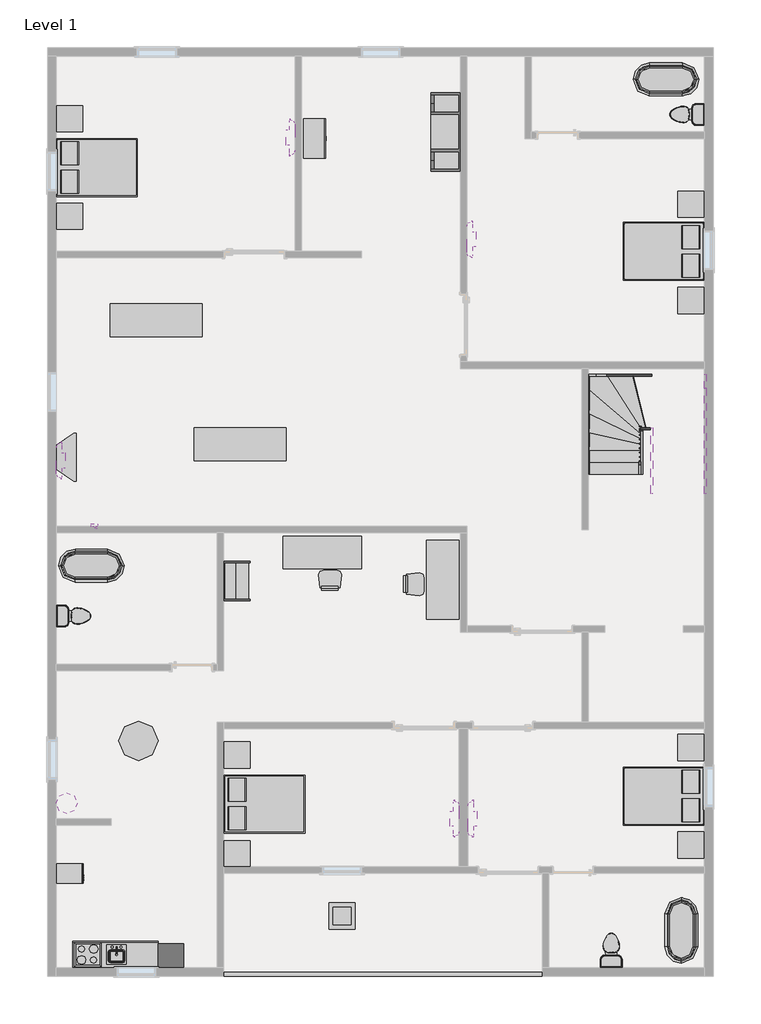
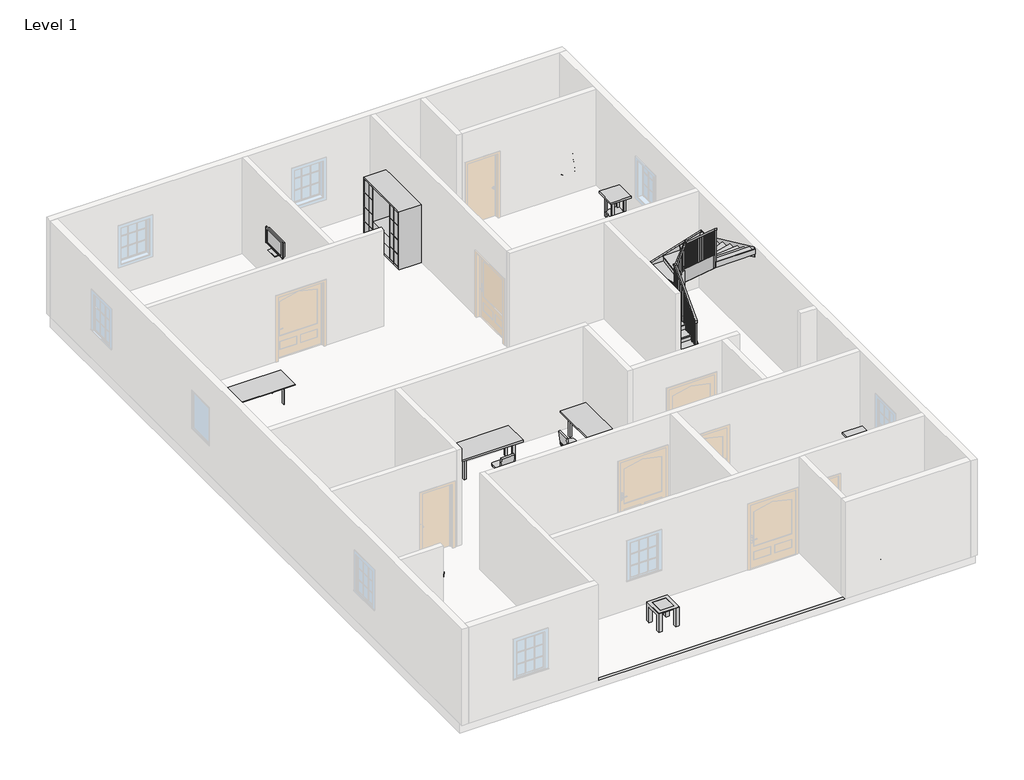
# One storey, part 2 of 2: 29 furniture elements, 9 members, 8 flow terminals, 8 proxies, 1 railing, 1 stair flight.
"""IFC4 building model written with IfcOpenShell, lengths in millimetres."""

from ifc_helpers import new_model, si_unit, frame, origin, place, context, project, spatial, polyline, outline, extrude, faceted_brep, triangles, transform, mapped, element, save
from components import proxy_7e1014cc, proxy_a6faaae8, proxy_45b28599, kitchenette_medium_kitchenette_medium_844211aa, rpc_picture_frame_rpc_picture_frame_c25e3fe9, proxy_c523a7b7, single_carrel_single_carrel_ed4d160c, flow_terminal_871c2e40, flow_terminal_d49f872f, toilet_domestic_3d_toilet_domestic_3d_f7549cf7, toilet_domestic_3d_toilet_domestic_3d_183bbd19, flow_terminal_b374fae2, furniture_c8abb964, chair_desk_chair_desk_ccc35c8f, furniture_c6510c7c, furniture_cf0b6580, furniture_e1dba61b, furniture_56245f3a, tv_stand_tv_stand_6ce107e5, furniture_b5c51a22, furniture_92191dda, furniture_905aceb5, furniture_5bc9ed15, furniture_a5b052b6, stair_flight_8a5f7a69

model = new_model("IFC4")

# Units and contexts
model_context = context("Model", 3, world=origin())
ifc_project = project(units=[si_unit("LENGTHUNIT", "METRE", prefix="MILLI")], contexts=[model_context])

# Site, building, storey
site = spatial("IfcSite", under=ifc_project)
building = spatial("IfcBuilding", under=site)
storey = spatial("IfcBuildingStorey", under=building, Name="Level 1", Elevation=0.0)

# Proxies
placement = place(None, origin())
element("IfcBuildingElementProxy", 1, Name="Building Element Proxy", at=placement, inside=storey, context=model_context, shape_type="Tessellation", body=[
    triangles([(-10823.7858398, -3895.8296448, 0.0), (-10823.7858398, -6283.4298386, 0.0), (-3432.3861305, -6283.4298386, 0.0), (-3432.3861305, -3895.8296448, 0.0)], [[1, 2, 4], [3, 4, 2]], closed=False),
])
proxy_shape = proxy_7e1014cc(model_context)
element("IfcBuildingElementProxy", 2, Name="18\" x 24\" x 34 1/2\"", ObjectType="18\" x 24\" x 34 1/2\"", at=placement, inside=storey, context=model_context, shape_type="MappedRepresentation", body=[
    mapped(proxy_shape, transform((-14138.7364865, -4201.9470633, 0.0), x_axis=(0.0, 1.0, 0.0), y_axis=(-1.0, 0.0, 0.0), z_axis=(0.0, 0.0, 1.0))),
])
proxy_2_shape = proxy_a6faaae8(model_context)
element("IfcBuildingElementProxy", 3, Name="Cook Top-4 Unit2 : 22\" x 20\"", ObjectType="Cook Top-4 Unit2 : 22\" x 20\"", at=placement, inside=storey, context=model_context, shape_type="MappedRepresentation", body=[
    mapped(proxy_2_shape, transform((-13986.0860513, -5775.4295948, 0.0), x_axis=(1.0, 0.0, 0.0), y_axis=(0.0, 1.0, 0.0), z_axis=(0.0, 0.0, 1.0))),
])
proxy_3_shape = proxy_45b28599(model_context)
element("IfcBuildingElementProxy", 4, Name="Dishwasher : 24\" x 24\" x 34\"", ObjectType="Dishwasher : 24\" x 24\" x 34\"", at=placement, inside=storey, context=model_context, shape_type="MappedRepresentation", body=[
    mapped(proxy_3_shape, transform((-13034.9035198, -6067.2791596, 0.0), x_axis=(1.0, 0.0, 0.0), y_axis=(0.0, 1.0, 0.0), z_axis=(0.0, 0.0, 1.0))),
])
kitchenette_medium_kitchenette_medium_shape = kitchenette_medium_kitchenette_medium_844211aa(model_context)
element("IfcBuildingElementProxy", 5, Name="Kitchenette - Medium : Kitchenette - Medium", ObjectType="Kitchenette - Medium : Kitchenette - Medium", at=placement, inside=storey, context=model_context, shape_type="MappedRepresentation", body=[
    mapped(kitchenette_medium_kitchenette_medium_shape, transform((-13661.9237562, -5470.6295948, 0.0), x_axis=(1.0, 0.0, 0.0), y_axis=(0.0, 1.0, 0.0), z_axis=(0.0, 0.0, 1.0))),
])
rpc_picture_frame_rpc_picture_frame_shape = rpc_picture_frame_rpc_picture_frame_c25e3fe9(model_context)
element("IfcBuildingElementProxy", 6, Name="RPC Picture Frame : RPC Picture Frame", ObjectType="RPC Picture Frame : RPC Picture Frame", at=placement, inside=storey, context=model_context, shape_type="MappedRepresentation", body=[
    mapped(rpc_picture_frame_rpc_picture_frame_shape, transform((-13828.5359953, 4155.9704052, 2133.6), x_axis=(-1.0000000000000004, 0.0, 0.0), y_axis=(0.0, -1.0000000000000004, 0.0), z_axis=(0.0, 0.0, 1.0))),
])
proxy_4_shape = proxy_c523a7b7(model_context)
element("IfcBuildingElementProxy", 7, Name="Refrigerator : 24\" x 25\" LH", ObjectType="Refrigerator : 24\" x 25\" LH", at=placement, inside=storey, context=model_context, shape_type="MappedRepresentation", body=[
    mapped(proxy_4_shape, transform((-12049.3360513, -5821.0785663, 0.0), x_axis=(1.0, 0.0, 0.0), y_axis=(0.0, 1.0, 0.0), z_axis=(0.0, 0.0, 1.0))),
])
single_carrel_single_carrel_shape = single_carrel_single_carrel_ed4d160c(model_context)
element("IfcBuildingElementProxy", 8, Name="Single Carrel : Single Carrel", ObjectType="Single Carrel : Single Carrel", at=placement, inside=storey, context=model_context, shape_type="MappedRepresentation", body=[
    mapped(single_carrel_single_carrel_shape, transform((-10823.7860513, 2885.9704052, 0.0), x_axis=(0.0, 1.0000000000000002, 0.0), y_axis=(-1.0000000000000002, 0.0, 0.0), z_axis=(0.0, 0.0, 1.0))),
])

# Flow terminals
flow_terminal_shape = flow_terminal_871c2e40(model_context)
element("IfcFlowTerminal", 9, ObjectType="Sink Kitchen-Island : 18\" x 18\"", at=placement, inside=storey, context=model_context, shape_type="MappedRepresentation", body=[
    mapped(flow_terminal_shape, transform((-13328.6752918, -5777.7749959, -14.4), x_axis=(1.0, 0.0, 0.0), y_axis=(0.0, 1.0, 0.0), z_axis=(0.0, 0.0, 1.0))),
])
flow_terminal_2_shape = flow_terminal_d49f872f(model_context)
element("IfcFlowTerminal", 10, ObjectType="Sink Vanity-Round : 19\" x 19\"", at=placement, inside=storey, context=model_context, shape_type="MappedRepresentation", body=[
    mapped(flow_terminal_2_shape, transform((-14385.2142446, -2366.8813354, 914.4), x_axis=(0.0, 1.0000000000000002, 0.0), y_axis=(-1.0000000000000002, 0.0, 0.0), z_axis=(0.0, 0.0, 1.0))),
])
toilet_domestic_3d_toilet_domestic_3d_shape = toilet_domestic_3d_toilet_domestic_3d_f7549cf7(model_context)
toilet_domestic_3d_toilet_domestic_3d_2_shape = toilet_domestic_3d_toilet_domestic_3d_183bbd19(model_context)
element("IfcFlowTerminal", 11, ObjectType="Toilet-Domestic-3D : Toilet-Domestic-3D", at=placement, inside=storey, context=model_context, shape_type="MappedRepresentation", body=[
    mapped(toilet_domestic_3d_toilet_domestic_3d_shape, transform((-1832.1860513, -5585.5335675, 0.0), x_axis=(-1.0000000000000004, 0.0, 0.0), y_axis=(0.0, -1.0000000000000004, 0.0), z_axis=(0.0, 0.0, 1.0))),
    mapped(toilet_domestic_3d_toilet_domestic_3d_2_shape, transform((-1832.1860513, -5585.5335675, 0.0), x_axis=(-1.0000000000000004, 0.0, 0.0), y_axis=(0.0, -1.0000000000000004, 0.0), z_axis=(0.0, 0.0, 1.0))),
])
element("IfcFlowTerminal", 12, ObjectType="Toilet-Domestic-3D : Toilet-Domestic-3D", at=placement, inside=storey, context=model_context, shape_type="MappedRepresentation", body=[
    mapped(toilet_domestic_3d_toilet_domestic_3d_shape, transform((-167.8820786, 13706.3704052, 0.0), x_axis=(0.0, -1.0000000000000002, 0.0), y_axis=(1.0000000000000002, 0.0, 0.0), z_axis=(0.0, 0.0, 1.0))),
    mapped(toilet_domestic_3d_toilet_domestic_3d_2_shape, transform((-167.8820786, 13706.3704052, 0.0), x_axis=(0.0, -1.0000000000000002, 0.0), y_axis=(1.0000000000000002, 0.0, 0.0), z_axis=(0.0, 0.0, 1.0))),
])
element("IfcFlowTerminal", 13, ObjectType="Toilet-Domestic-3D : Toilet-Domestic-3D", at=placement, inside=storey, context=model_context, shape_type="MappedRepresentation", body=[
    mapped(toilet_domestic_3d_toilet_domestic_3d_shape, transform((-14215.2900239, 2073.1704052, 0.0), x_axis=(0.0, 1.0000000000000002, 0.0), y_axis=(-1.0000000000000002, 0.0, 0.0), z_axis=(0.0, 0.0, 1.0))),
    mapped(toilet_domestic_3d_toilet_domestic_3d_2_shape, transform((-14215.2900239, 2073.1704052, 0.0), x_axis=(0.0, 1.0000000000000002, 0.0), y_axis=(-1.0000000000000002, 0.0, 0.0), z_axis=(0.0, 0.0, 1.0))),
])
flow_terminal_3_shape = flow_terminal_b374fae2(model_context)
element("IfcFlowTerminal", 14, ObjectType="Tub-Free Standing-3D : 30\" x 60\"", at=placement, inside=storey, context=model_context, shape_type="MappedRepresentation", body=[
    mapped(flow_terminal_3_shape, transform((-206.5860513, -5216.6295948, 0.0), x_axis=(-1.0000000000000004, 0.0, 0.0), y_axis=(0.0, -1.0000000000000004, 0.0), z_axis=(0.0, 0.0, 1.0))),
])
element("IfcFlowTerminal", 15, ObjectType="Tub-Free Standing-3D : 30\" x 60\"", at=placement, inside=storey, context=model_context, shape_type="MappedRepresentation", body=[
    mapped(flow_terminal_3_shape, transform((-13897.1860513, 3241.5704052, 0.0), x_axis=(0.0, 1.0000000000000004, 0.0), y_axis=(-1.0000000000000004, 0.0, 0.0), z_axis=(0.0, 0.0, 1.0))),
])
element("IfcFlowTerminal", 16, ObjectType="Tub-Free Standing-3D : 30\" x 60\"", at=placement, inside=storey, context=model_context, shape_type="MappedRepresentation", body=[
    mapped(flow_terminal_3_shape, transform((-562.1860513, 14519.1704052, 0.0), x_axis=(0.0, -1.0000000000000004, 0.0), y_axis=(1.0000000000000004, 0.0, 0.0), z_axis=(0.0, 0.0, 1.0))),
])

# Furniture
furniture_shape = furniture_c8abb964(model_context)
element("IfcFurniture", 17, ObjectType="Bed-Box : Double 53\" x 74\"", at=placement, inside=storey, context=model_context, shape_type="MappedRepresentation", body=[
    mapped(furniture_shape, transform((-10118.4155595, -2625.8295948, 0.0), x_axis=(0.0, 1.0, 0.0), y_axis=(-1.0, 0.0, 0.0), z_axis=(0.0, 0.0, 1.0))),
])
element("IfcFurniture", 18, ObjectType="Bed-Box : Double 53\" x 74\"", at=placement, inside=storey, context=model_context, shape_type="MappedRepresentation", body=[
    mapped(furniture_shape, transform((-378.5565431, -1765.9771358, 0.0), x_axis=(0.0, -1.0000000000000004, 0.0), y_axis=(1.0000000000000004, 0.0, 0.0), z_axis=(0.0, 0.0, 1.0))),
])
element("IfcFurniture", 19, ObjectType="Bed-Box : Double 53\" x 74\"", at=placement, inside=storey, context=model_context, shape_type="MappedRepresentation", body=[
    mapped(furniture_shape, transform((-14004.6155595, 12135.3179462, 0.0), x_axis=(0.0, 1.0000000000000007, 0.0), y_axis=(-1.0000000000000007, 0.0, 0.0), z_axis=(0.0, 0.0, 1.0))),
])
element("IfcFurniture", 20, ObjectType="Bed-Box : Double 53\" x 74\"", at=placement, inside=storey, context=model_context, shape_type="MappedRepresentation", body=[
    mapped(furniture_shape, transform((-378.5565431, 10870.5228642, 0.0), x_axis=(0.0, -1.0000000000000004, 0.0), y_axis=(1.0000000000000004, 0.0, 0.0), z_axis=(0.0, 0.0, 1.0))),
])
chair_desk_chair_desk_shape = chair_desk_chair_desk_ccc35c8f(model_context)
element("IfcFurniture", 21, ObjectType="Chair-Desk : Chair-Desk", at=placement, inside=storey, context=model_context, shape_type="MappedRepresentation", body=[
    mapped(chair_desk_chair_desk_shape, transform((-8359.9860513, 2733.5704052, 0.0), x_axis=(1.0, 0.0, 0.0), y_axis=(0.0, 1.0, 0.0), z_axis=(0.0, 0.0, 1.0))),
])
element("IfcFurniture", 22, ObjectType="Chair-Desk : Chair-Desk", at=placement, inside=storey, context=model_context, shape_type="MappedRepresentation", body=[
    mapped(chair_desk_chair_desk_shape, transform((-6581.9860513, 2809.7704052, 0.0), x_axis=(0.0, -1.0000000000000004, 0.0), y_axis=(1.0000000000000004, 0.0, 0.0), z_axis=(0.0, 0.0, 1.0))),
])
furniture_2_shape = furniture_c6510c7c(model_context)
element("IfcFurniture", 23, ObjectType="Counter Top w Sink Hole : 24\" Depth", at=placement, inside=storey, context=model_context, shape_type="MappedRepresentation", body=[
    mapped(furniture_2_shape, transform((-13128.5237562, -5470.6295948, -14.4), x_axis=(1.0, 0.0, 0.0), y_axis=(0.0, 1.0, 0.0), z_axis=(0.0, 0.0, 1.0))),
])
furniture_3_shape = furniture_cf0b6580(model_context)
element("IfcFurniture", 24, ObjectType="Entertainment Center : 72\" x 72\" x 24\"", at=placement, inside=storey, context=model_context, shape_type="MappedRepresentation", body=[
    mapped(furniture_3_shape, transform((-5235.7860513, 13299.9704052, 0.0), x_axis=(0.0, -1.0000000000000007, 0.0), y_axis=(1.0000000000000007, 0.0, 0.0), z_axis=(0.0, 0.0, 1.0))),
])
furniture_4_shape = furniture_e1dba61b(model_context)
element("IfcFurniture", 25, ObjectType="Storage Pedestal : 20\" x 36\" x 36\"", at=placement, inside=storey, context=model_context, shape_type="MappedRepresentation", body=[
    mapped(furniture_4_shape, transform((-9649.9044273, 13327.5929191, 0.0), x_axis=(0.0, 1.0000000000000009, 0.0), y_axis=(-1.0000000000000009, 0.0, 0.0), z_axis=(0.0, 0.0, 1.0))),
])
furniture_5_shape = furniture_56245f3a(model_context)
element("IfcFurniture", 26, ObjectType="TV - Flat Screen : 32\"", at=placement, inside=storey, context=model_context, shape_type="MappedRepresentation", body=[
    mapped(furniture_5_shape, transform((-14651.4474276, 5683.9149193, 1524.0), x_axis=(0.0, 1.0000000000000002, 0.0), y_axis=(-1.0000000000000002, 0.0, 0.0), z_axis=(0.0, 0.0, 1.0))),
])
element("IfcFurniture", 27, ObjectType="TV - Flat Screen : 32\"", at=placement, inside=storey, context=model_context, shape_type="MappedRepresentation", body=[
    mapped(furniture_5_shape, transform((-5101.0474276, -2621.8850807, 1219.2), x_axis=(0.0, 1.0000000000000002, 0.0), y_axis=(-1.0000000000000002, 0.0, 0.0), z_axis=(0.0, 0.0, 1.0))),
])
element("IfcFurniture", 28, ObjectType="TV - Flat Screen : 32\"", at=placement, inside=storey, context=model_context, shape_type="MappedRepresentation", body=[
    mapped(furniture_5_shape, transform((-5421.3246749, -2629.774109, 1219.2), x_axis=(0.0, -1.0000000000000002, 0.0), y_axis=(1.0000000000000002, 0.0, 0.0), z_axis=(0.0, 0.0, 1.0))),
])
element("IfcFurniture", 29, ObjectType="TV - Flat Screen : 32\"", at=placement, inside=storey, context=model_context, shape_type="MappedRepresentation", body=[
    mapped(furniture_5_shape, transform((-5126.4474276, 10814.7149193, 1219.2), x_axis=(0.0, 1.0000000000000002, 0.0), y_axis=(-1.0000000000000002, 0.0, 0.0), z_axis=(0.0, 0.0, 1.0))),
])
element("IfcFurniture", 30, ObjectType="TV - Flat Screen : 32\"", at=placement, inside=storey, context=model_context, shape_type="MappedRepresentation", body=[
    mapped(furniture_5_shape, transform((-9231.3246749, 13169.025891, 1219.2), x_axis=(0.0, -1.0000000000000004, 0.0), y_axis=(1.0000000000000004, 0.0, 0.0), z_axis=(0.0, 0.0, 1.0))),
])
tv_stand_tv_stand_shape = tv_stand_tv_stand_6ce107e5(model_context)
element("IfcFurniture", 31, ObjectType="TV Stand : TV Stand", at=placement, inside=storey, context=model_context, shape_type="MappedRepresentation", body=[
    mapped(tv_stand_tv_stand_shape, transform((-14709.9860513, 5630.9824031, 0.0), x_axis=(0.0, 1.0000000000000002, 0.0), y_axis=(-1.0000000000000002, 0.0, 0.0), z_axis=(0.0, 0.0, 1.0))),
])
furniture_6_shape = furniture_b5c51a22(model_context)
element("IfcFurniture", 32, ObjectType="Table-Coffee : 24\" x 24\" x 24\"", at=placement, inside=storey, context=model_context, shape_type="MappedRepresentation", body=[
    mapped(furniture_6_shape, transform((-8098.8518179, -4981.6406726, 0.0), x_axis=(1.0, 0.0, 0.0), y_axis=(0.0, 1.0, 0.0), z_axis=(0.0, 0.0, 1.0))),
])
furniture_7_shape = furniture_92191dda(model_context)
element("IfcFurniture", 33, ObjectType="Table-Dining : 30\" x 84\" x 22\"", at=placement, inside=storey, context=model_context, shape_type="MappedRepresentation", body=[
    mapped(furniture_7_shape, transform((-10461.0518179, 5965.7593274, 0.0), x_axis=(1.0, 0.0, 0.0), y_axis=(0.0, 1.0, 0.0), z_axis=(0.0, 0.0, 1.0))),
])
element("IfcFurniture", 34, ObjectType="Table-Dining : 30\" x 84\" x 22\"", at=placement, inside=storey, context=model_context, shape_type="MappedRepresentation", body=[
    mapped(furniture_7_shape, transform((-12416.8518179, 8835.9593274, 0.0), x_axis=(1.0, 0.0, 0.0), y_axis=(0.0, 1.0, 0.0), z_axis=(0.0, 0.0, 1.0))),
])
furniture_8_shape = furniture_905aceb5(model_context)
element("IfcFurniture", 35, ObjectType="Table-Dining Round w Chairs : 36\" Diameter", at=placement, inside=storey, context=model_context, shape_type="MappedRepresentation", body=[
    mapped(furniture_8_shape, transform((-12908.6680185, -637.5509063, 0.0), x_axis=(1.0, 0.0, 0.0), y_axis=(0.0, 1.0, 0.0), z_axis=(0.0, 0.0, 1.0))),
])
furniture_9_shape = furniture_5bc9ed15(model_context)
element("IfcFurniture", 36, ObjectType="Table-Night Stand : 24\" x 24\" x 30\"", at=placement, inside=storey, context=model_context, shape_type="MappedRepresentation", body=[
    mapped(furniture_9_shape, transform((-10827.5196816, -3743.4295948, 0.0), x_axis=(1.0, 0.0, 0.0), y_axis=(0.0, 1.0, 0.0), z_axis=(0.0, 0.0, 1.0))),
])
element("IfcFurniture", 37, ObjectType="Table-Night Stand : 24\" x 24\" x 30\"", at=placement, inside=storey, context=model_context, shape_type="MappedRepresentation", body=[
    mapped(furniture_9_shape, transform((-10827.5196816, -1457.4295948, 0.0), x_axis=(1.0, 0.0, 0.0), y_axis=(0.0, 1.0, 0.0), z_axis=(0.0, 0.0, 1.0))),
])
element("IfcFurniture", 38, ObjectType="Table-Night Stand : 24\" x 24\" x 30\"", at=placement, inside=storey, context=model_context, shape_type="MappedRepresentation", body=[
    mapped(furniture_9_shape, transform((-286.5196816, -3540.2295948, 0.0), x_axis=(1.0, 0.0, 0.0), y_axis=(0.0, 1.0, 0.0), z_axis=(0.0, 0.0, 1.0))),
])
element("IfcFurniture", 39, ObjectType="Table-Night Stand : 24\" x 24\" x 30\"", at=placement, inside=storey, context=model_context, shape_type="MappedRepresentation", body=[
    mapped(furniture_9_shape, transform((-286.5196816, -1279.6295948, 0.0), x_axis=(1.0, 0.0, 0.0), y_axis=(0.0, 1.0, 0.0), z_axis=(0.0, 0.0, 1.0))),
])
element("IfcFurniture", 40, ObjectType="Table-Night Stand : 24\" x 24\" x 30\"", at=placement, inside=storey, context=model_context, shape_type="MappedRepresentation", body=[
    mapped(furniture_9_shape, transform((-286.5196816, 11318.7704052, 0.0), x_axis=(1.0, 0.0, 0.0), y_axis=(0.0, 1.0, 0.0), z_axis=(0.0, 0.0, 1.0))),
])
element("IfcFurniture", 41, ObjectType="Table-Night Stand : 24\" x 24\" x 30\"", at=placement, inside=storey, context=model_context, shape_type="MappedRepresentation", body=[
    mapped(furniture_9_shape, transform((-286.5196816, 9083.5704052, 0.0), x_axis=(1.0, 0.0, 0.0), y_axis=(0.0, 1.0, 0.0), z_axis=(0.0, 0.0, 1.0))),
])
element("IfcFurniture", 42, ObjectType="Table-Night Stand : 24\" x 24\" x 30\"", at=placement, inside=storey, context=model_context, shape_type="MappedRepresentation", body=[
    mapped(furniture_9_shape, transform((-14713.7196816, 13299.9704052, 0.0), x_axis=(1.0, 0.0, 0.0), y_axis=(0.0, 1.0, 0.0), z_axis=(0.0, 0.0, 1.0))),
])
element("IfcFurniture", 43, ObjectType="Table-Night Stand : 24\" x 24\" x 30\"", at=placement, inside=storey, context=model_context, shape_type="MappedRepresentation", body=[
    mapped(furniture_9_shape, transform((-14713.7196816, 11039.3704052, 0.0), x_axis=(1.0, 0.0, 0.0), y_axis=(0.0, 1.0, 0.0), z_axis=(0.0, 0.0, 1.0))),
])
furniture_10_shape = furniture_a5b052b6(model_context)
element("IfcFurniture", 44, ObjectType="Table-Rectangular : 72\" x 30\"", at=placement, inside=storey, context=model_context, shape_type="MappedRepresentation", body=[
    mapped(furniture_10_shape, transform((-8537.7860513, 3546.3704052, 0.0), x_axis=(1.0, 0.0, 0.0), y_axis=(0.0, 1.0, 0.0), z_axis=(0.0, 0.0, 1.0))),
])
element("IfcFurniture", 45, ObjectType="Table-Rectangular : 72\" x 30\"", at=placement, inside=storey, context=model_context, shape_type="MappedRepresentation", body=[
    mapped(furniture_10_shape, transform((-5743.7860513, 2911.3704052, 0.0), x_axis=(0.0, -1.0000000000000004, 0.0), y_axis=(1.0000000000000004, 0.0, 0.0), z_axis=(0.0, 0.0, 1.0))),
])

# Members
element("IfcMember", 46, ObjectType="Stringer - 2\" Width", at=placement, inside=storey, context=model_context, shape_type="SweptSolid", body=[
    extrude(outline(polyline([(5356.2607598, 0.0), (5356.2607598, 253.7697654), (7536.5486445, 1127.7715314), (7536.5486445, 799.3938411), (5542.377952, 0.0), (5356.2607598, 0.0)])), frame((-2389.7053008, 0.0, 0.0), z_axis=(1.0, 0.0, 0.0), x_axis=(0.0, 1.0, 0.0)), (0.0, 0.0, 1.0), 50.8),
])
element("IfcMember", 47, ObjectType="Stringer - 2\" Width", at=placement, inside=storey, context=model_context, shape_type="SweptSolid", body=[
    extrude(outline(polyline([(-2338.9053008, 7536.5486445), (-2389.7053008, 7536.5486445), (-2389.7053008, 7685.2896548), (-2338.9053008, 7634.4896548), (-2338.9053008, 7536.5486445)])), frame((0.0, 0.0, 799.3938411), z_axis=(0.0, 0.0, 1.0), x_axis=(1.0, 0.0, 0.0)), (0.0, 0.0, 1.0), 328.3776903),
])
element("IfcMember", 48, ObjectType="Stringer - 2\" Width", at=placement, inside=storey, context=model_context, shape_type="SweptSolid", body=[
    extrude(outline(polyline([(-2338.9053008, 7634.4896548), (-2389.7053008, 7685.2896548), (-2181.2813511, 7685.2896548), (-2181.2813511, 7634.4896548), (-2338.9053008, 7634.4896548)])), frame((0.0, 0.0, 799.3938411), z_axis=(0.0, 0.0, 1.0), x_axis=(1.0, 0.0, 0.0)), (0.0, 0.0, 1.0), 328.3776903),
])
element("IfcMember", 49, ObjectType="Stringer - 2\" Width", at=placement, inside=storey, context=model_context, shape_type="SweptSolid", body=[
    extrude(outline(polyline([(1127.7715314, -2181.2813511), (799.3938411, -2181.2813511), (1575.7906145, 325.5331983), (1899.7048199, 325.5331983), (1899.7048199, 311.1215864), (1127.7715314, -2181.2813511)])), frame((0.0, 7634.4896548, 0.0), z_axis=(0.0, 1.0, 0.0), x_axis=(0.0, 0.0, 1.0)), (0.0, 0.0, 1.0), 50.8),
])
element("IfcMember", 50, ObjectType="Stringer - 2\" Width", at=placement, inside=storey, context=model_context, shape_type="SweptSolid", body=[
    extrude(outline(polyline([(325.5331983, 7685.2896548), (376.3331983, 7685.2896548), (376.3331983, 7355.703067), (325.5331983, 7355.703067), (325.5331983, 7685.2896548)])), frame((0.0, 0.0, 1580.6208435), z_axis=(0.0, 0.0, 1.0), x_axis=(1.0, 0.0, 0.0)), (0.0, 0.0, 1.0), 319.0839764),
])
element("IfcMember", 51, ObjectType="Stringer - 2\" Width", at=placement, inside=storey, context=model_context, shape_type="SweptSolid", body=[
    extrude(outline(polyline([(5356.2607598, 0.0), (5356.2607598, 140.6708409), (6391.1704052, 1235.2332807), (6391.1704052, 791.5839653), (5642.7271451, 0.0), (5356.2607598, 0.0)])), frame((-1146.3860513, 0.0, 0.0), z_axis=(1.0, 0.0, 0.0), x_axis=(0.0, 1.0, 0.0)), (0.0, 0.0, 1.0), 50.8),
])
element("IfcMember", 52, ObjectType="Stringer - 2\" Width", at=placement, inside=storey, context=model_context, shape_type="SweptSolid", body=[
    extrude(outline(polyline([(1453.6314878, -1146.3860513), (845.3121069, -1146.3860513), (845.3121069, -1087.3182945), (1219.5911959, -917.7860513), (1835.3677632, -917.7860513), (1835.3677632, -973.4760251), (1453.6314878, -1146.3860513)])), frame((0.0, 6391.1704052, 0.0), z_axis=(0.0, 1.0, 0.0), x_axis=(0.0, 0.0, 1.0)), (0.0, 0.0, 1.0), 50.8),
])
element("IfcMember", 53, ObjectType="Stringer - 2\" Width", at=placement, inside=storey, context=model_context, shape_type="SweptSolid", body=[
    extrude(outline(polyline([(6441.9704052, 1835.3677632), (6441.9704052, 1426.0789229), (4914.2387133, 2795.2042452), (4914.2387133, 3204.4930856), (6441.9704052, 1835.3677632)])), frame((-917.7860513, 0.0, 0.0), z_axis=(1.0, 0.0, 0.0), x_axis=(0.0, 1.0, 0.0)), (0.0, 0.0, 1.0), 50.8),
])
element("IfcMember", 54, ObjectType="Stringer - 2\" Width", at=placement, inside=storey, context=model_context, shape_type="SweptSolid", body=[
    extrude(outline(polyline([(7355.703067, 1899.7048199), (7355.703067, 1580.6208435), (4914.2387133, 2711.6595982), (4914.2387133, 3030.7435746), (7355.703067, 1899.7048199)])), frame((325.5331983, 0.0, 0.0), z_axis=(1.0, 0.0, 0.0), x_axis=(0.0, 1.0, 0.0)), (0.0, 0.0, 1.0), 50.8),
])

# Railing
element("IfcRailing", 55, ObjectType="Handrail - Rectangular", at=placement, inside=storey, context=model_context, shape_type="SolidModel", body=[
    faceted_brep([(-1197.1860513, 5356.2607598, 957.561888), (-1197.1860513, 5356.2607598, 883.6203354), (-1146.3860513, 5356.2607598, 883.6203354), (-1146.3860513, 5356.2607598, 957.561888), (-1197.1860513, 6412.8357789, 2075.0385063), (-1197.1860513, 6434.716135, 2024.2385063), (-1146.3860513, 6434.716135, 2024.2385063), (-1146.3860513, 6412.8357789, 2075.0385063), (-1197.1860513, 6492.7704052, 2075.0385063), (-1146.3860513, 6492.7704052, 2075.0385063), (-1146.3860513, 6492.7704052, 2024.2385063), (-1197.1860513, 6492.7704052, 2024.2385063)], [[[0, 1, 2, 3]], [[1, 0, 4, 5]], [[2, 1, 5, 6]], [[3, 2, 6, 7]], [[0, 3, 7, 4]], [[8, 9, 10, 11]], [[5, 4, 8, 11]], [[6, 5, 11, 10]], [[7, 6, 10, 9]], [[4, 7, 9, 8]]]),
    faceted_brep([(-1146.3860513, 6492.7704052, 2073.4364653), (-1146.3860513, 6492.7704052, 1950.3157607), (-1146.3860513, 6441.9704052, 1950.3157607), (-1146.3860513, 6441.9704052, 2073.4364653), (-866.9860513, 6492.7704052, 2690.2723869), (-866.9860513, 6441.9704052, 2690.2723869), (-866.9860513, 6441.9704052, 2567.1516822), (-866.9860513, 6492.7704052, 2567.1516822)], [[[0, 1, 2, 3]], [[4, 5, 6, 7]], [[1, 0, 4, 7]], [[2, 1, 7, 6]], [[3, 2, 6, 5]], [[0, 3, 5, 4]]]),
    faceted_brep([(-816.1860513, 6492.7704052, 2698.9599494), (-816.1860513, 6492.7704052, 2648.1599494), (-866.9860513, 6492.7704052, 2648.1599494), (-866.9860513, 6492.7704052, 2698.9599494), (-816.1860513, 6414.4922605, 2698.9599494), (-816.1860513, 6395.0600349, 2648.1599494), (-866.9860513, 6395.0600349, 2648.1599494), (-866.9860513, 6414.4922605, 2698.9599494), (-816.1860513, 4914.2387133, 4043.4598588), (-866.9860513, 4914.2387133, 4043.4598588), (-866.9860513, 4914.2387133, 3975.2450521), (-816.1860513, 4914.2387133, 3975.2450521)], [[[0, 1, 2, 3]], [[1, 0, 4, 5]], [[2, 1, 5, 6]], [[3, 2, 6, 7]], [[0, 3, 7, 4]], [[8, 9, 10, 11]], [[5, 4, 8, 11]], [[6, 5, 11, 10]], [[7, 6, 10, 9]], [[4, 7, 9, 8]]]),
    extrude(outline(polyline([(4982.5672605, 3914.0102524), (5001.6172605, 3896.9379893), (5001.6172605, 2878.6666667), (4982.5672605, 2878.6666667), (4982.5672605, 3914.0102524)])), frame((-851.1110513, 0.0, 0.0), z_axis=(1.0, 0.0, 0.0), x_axis=(0.0, 1.0, 0.0)), (0.0, 0.0, 1.0), 19.05),
    extrude(outline(polyline([(5084.1672605, 3822.9581825), (5103.2172605, 3805.8859194), (5103.2172605, 2878.6666667), (5084.1672605, 2878.6666667), (5084.1672605, 3822.9581825)])), frame((-851.1110513, 0.0, 0.0), z_axis=(1.0, 0.0, 0.0), x_axis=(0.0, 1.0, 0.0)), (0.0, 0.0, 1.0), 19.05),
    extrude(outline(polyline([(5185.7672605, 3731.9061126), (5204.8172605, 3714.8338495), (5204.8172605, 2709.3333333), (5185.7672605, 2709.3333333), (5185.7672605, 3731.9061126)])), frame((-851.1110513, 0.0, 0.0), z_axis=(1.0, 0.0, 0.0), x_axis=(0.0, 1.0, 0.0)), (0.0, 0.0, 1.0), 19.05),
    extrude(outline(polyline([(5287.3672605, 3640.8540428), (5306.4172605, 3623.7817797), (5306.4172605, 2709.3333333), (5287.3672605, 2709.3333333), (5287.3672605, 3640.8540428)])), frame((-851.1110513, 0.0, 0.0), z_axis=(1.0, 0.0, 0.0), x_axis=(0.0, 1.0, 0.0)), (0.0, 0.0, 1.0), 19.05),
    extrude(outline(polyline([(5388.9672605, 3549.8019729), (5408.0172605, 3532.7297098), (5408.0172605, 2709.3333333), (5388.9672605, 2709.3333333), (5388.9672605, 3549.8019729)])), frame((-851.1110513, 0.0, 0.0), z_axis=(1.0, 0.0, 0.0), x_axis=(0.0, 1.0, 0.0)), (0.0, 0.0, 1.0), 19.05),
    extrude(outline(polyline([(5490.5672605, 3458.749903), (5509.6172605, 3441.6776399), (5509.6172605, 2540.0), (5490.5672605, 2540.0), (5490.5672605, 3458.749903)])), frame((-851.1110513, 0.0, 0.0), z_axis=(1.0, 0.0, 0.0), x_axis=(0.0, 1.0, 0.0)), (0.0, 0.0, 1.0), 19.05),
    extrude(outline(polyline([(5592.1672605, 3367.6978332), (5611.2172605, 3350.6255701), (5611.2172605, 2540.0), (5592.1672605, 2540.0), (5592.1672605, 3367.6978332)])), frame((-851.1110513, 0.0, 0.0), z_axis=(1.0, 0.0, 0.0), x_axis=(0.0, 1.0, 0.0)), (0.0, 0.0, 1.0), 19.05),
    extrude(outline(polyline([(5693.7672605, 3276.6457633), (5712.8172605, 3259.5735002), (5712.8172605, 2370.6666667), (5693.7672605, 2370.6666667), (5693.7672605, 3276.6457633)])), frame((-851.1110513, 0.0, 0.0), z_axis=(1.0, 0.0, 0.0), x_axis=(0.0, 1.0, 0.0)), (0.0, 0.0, 1.0), 19.05),
    extrude(outline(polyline([(5795.3672605, 3185.5936934), (5814.4172605, 3168.5214303), (5814.4172605, 2370.6666667), (5795.3672605, 2370.6666667), (5795.3672605, 3185.5936934)])), frame((-851.1110513, 0.0, 0.0), z_axis=(1.0, 0.0, 0.0), x_axis=(0.0, 1.0, 0.0)), (0.0, 0.0, 1.0), 19.05),
    extrude(outline(polyline([(5896.9672605, 3094.5416235), (5916.0172605, 3077.4693604), (5916.0172605, 2201.3333333), (5896.9672605, 2201.3333333), (5896.9672605, 3094.5416235)])), frame((-851.1110513, 0.0, 0.0), z_axis=(1.0, 0.0, 0.0), x_axis=(0.0, 1.0, 0.0)), (0.0, 0.0, 1.0), 19.05),
    extrude(outline(polyline([(5998.5672605, 3003.4895537), (6017.6172605, 2986.4172906), (6017.6172605, 2201.3333333), (5998.5672605, 2201.3333333), (5998.5672605, 3003.4895537)])), frame((-851.1110513, 0.0, 0.0), z_axis=(1.0, 0.0, 0.0), x_axis=(0.0, 1.0, 0.0)), (0.0, 0.0, 1.0), 19.05),
    extrude(outline(polyline([(6100.1672605, 2912.4374838), (6119.2172605, 2895.3652207), (6119.2172605, 2032.0), (6100.1672605, 2032.0), (6100.1672605, 2912.4374838)])), frame((-851.1110513, 0.0, 0.0), z_axis=(1.0, 0.0, 0.0), x_axis=(0.0, 1.0, 0.0)), (0.0, 0.0, 1.0), 19.05),
    extrude(outline(polyline([(6201.7672605, 2821.3854139), (6220.8172605, 2804.3131508), (6220.8172605, 1862.6666667), (6201.7672605, 1862.6666667), (6201.7672605, 2821.3854139)])), frame((-851.1110513, 0.0, 0.0), z_axis=(1.0, 0.0, 0.0), x_axis=(0.0, 1.0, 0.0)), (0.0, 0.0, 1.0), 19.05),
    extrude(outline(polyline([(6303.3672605, 2730.333344), (6322.4172605, 2713.2610809), (6322.4172605, 1862.6666667), (6303.3672605, 1862.6666667), (6303.3672605, 2730.333344)])), frame((-851.1110513, 0.0, 0.0), z_axis=(1.0, 0.0, 0.0), x_axis=(0.0, 1.0, 0.0)), (0.0, 0.0, 1.0), 19.05),
    extrude(outline(polyline([(2421.554242, -932.935396), (2379.4972473, -951.985396), (1524.0, -951.985396), (1524.0, -932.935396), (2421.554242, -932.935396)])), frame((0.0, 6457.8454052, 0.0), z_axis=(0.0, 1.0, 0.0), x_axis=(0.0, 0.0, 1.0)), (0.0, 0.0, 1.0), 19.05),
    extrude(outline(polyline([(2197.2502705, -1034.535396), (2155.1932759, -1053.585396), (1354.6666667, -1053.585396), (1354.6666667, -1034.535396), (2197.2502705, -1034.535396)])), frame((0.0, 6457.8454052, 0.0), z_axis=(0.0, 1.0, 0.0), x_axis=(0.0, 0.0, 1.0)), (0.0, 0.0, 1.0), 19.05),
    extrude(outline(polyline([(6362.7357598, 1948.1091404), (6381.7857598, 1968.2571935), (6381.7857598, 1016.0), (6362.7357598, 1016.0), (6362.7357598, 1948.1091404)])), frame((-1181.3110513, 0.0, 0.0), z_axis=(1.0, 0.0, 0.0), x_axis=(0.0, 1.0, 0.0)), (0.0, 0.0, 1.0), 19.05),
    extrude(outline(polyline([(6261.1357598, 1840.6528572), (6280.1857598, 1860.8009103), (6280.1857598, 846.6666667), (6261.1357598, 846.6666667), (6261.1357598, 1840.6528572)])), frame((-1181.3110513, 0.0, 0.0), z_axis=(1.0, 0.0, 0.0), x_axis=(0.0, 1.0, 0.0)), (0.0, 0.0, 1.0), 19.05),
    extrude(outline(polyline([(6159.5357598, 1733.1965741), (6178.5857598, 1753.3446272), (6178.5857598, 677.3333333), (6159.5357598, 677.3333333), (6159.5357598, 1733.1965741)])), frame((-1181.3110513, 0.0, 0.0), z_axis=(1.0, 0.0, 0.0), x_axis=(0.0, 1.0, 0.0)), (0.0, 0.0, 1.0), 19.05),
    extrude(outline(polyline([(6057.9357598, 1625.7402909), (6076.9857598, 1645.888344), (6076.9857598, 508.0), (6057.9357598, 508.0), (6057.9357598, 1625.7402909)])), frame((-1181.3110513, 0.0, 0.0), z_axis=(1.0, 0.0, 0.0), x_axis=(0.0, 1.0, 0.0)), (0.0, 0.0, 1.0), 19.05),
    extrude(outline(polyline([(5956.3357598, 1518.2840078), (5975.3857598, 1538.4320609), (5975.3857598, 508.0), (5956.3357598, 508.0), (5956.3357598, 1518.2840078)])), frame((-1181.3110513, 0.0, 0.0), z_axis=(1.0, 0.0, 0.0), x_axis=(0.0, 1.0, 0.0)), (0.0, 0.0, 1.0), 19.05),
    extrude(outline(polyline([(5854.7357598, 1410.8277246), (5873.7857598, 1430.9757777), (5873.7857598, 338.6666667), (5854.7357598, 338.6666667), (5854.7357598, 1410.8277246)])), frame((-1181.3110513, 0.0, 0.0), z_axis=(1.0, 0.0, 0.0), x_axis=(0.0, 1.0, 0.0)), (0.0, 0.0, 1.0), 19.05),
    extrude(outline(polyline([(5753.1357598, 1303.3714415), (5772.1857598, 1323.5194946), (5772.1857598, 338.6666667), (5753.1357598, 338.6666667), (5753.1357598, 1303.3714415)])), frame((-1181.3110513, 0.0, 0.0), z_axis=(1.0, 0.0, 0.0), x_axis=(0.0, 1.0, 0.0)), (0.0, 0.0, 1.0), 19.05),
    extrude(outline(polyline([(5651.5357598, 1195.9151583), (5670.5857598, 1216.0632114), (5670.5857598, 338.6666667), (5651.5357598, 338.6666667), (5651.5357598, 1195.9151583)])), frame((-1181.3110513, 0.0, 0.0), z_axis=(1.0, 0.0, 0.0), x_axis=(0.0, 1.0, 0.0)), (0.0, 0.0, 1.0), 19.05),
    extrude(outline(polyline([(5549.9357598, 1088.4588752), (5568.9857598, 1108.6069283), (5568.9857598, 169.3333333), (5549.9357598, 169.3333333), (5549.9357598, 1088.4588752)])), frame((-1181.3110513, 0.0, 0.0), z_axis=(1.0, 0.0, 0.0), x_axis=(0.0, 1.0, 0.0)), (0.0, 0.0, 1.0), 19.05),
    extrude(outline(polyline([(5448.3357598, 981.002592), (5467.3857598, 1001.1506451), (5467.3857598, 169.3333333), (5448.3357598, 169.3333333), (5448.3357598, 981.002592)])), frame((-1181.3110513, 0.0, 0.0), z_axis=(1.0, 0.0, 0.0), x_axis=(0.0, 1.0, 0.0)), (0.0, 0.0, 1.0), 19.05),
    extrude(outline(polyline([(-851.1110513, 6424.0172605), (-832.0610513, 6424.0172605), (-832.0610513, 6404.9672605), (-851.1110513, 6404.9672605), (-851.1110513, 6424.0172605)])), frame((0.0, 0.0, 1693.3333333), z_axis=(0.0, 0.0, 1.0), x_axis=(1.0, 0.0, 0.0)), (0.0, 0.0, 1.0), 954.826616),
    extrude(outline(polyline([(2644.2561724, -832.0610513), (2602.1991778, -851.1110513), (1693.3333333, -851.1110513), (1693.3333333, -832.0610513), (2644.2561724, -832.0610513)])), frame((0.0, 6457.8454052, 0.0), z_axis=(0.0, 1.0, 0.0), x_axis=(0.0, 0.0, 1.0)), (0.0, 0.0, 1.0), 19.05),
    extrude(outline(polyline([(2596.8677421, -853.5259611), (2554.8107474, -872.5759611), (1693.3333333, -872.5759611), (1693.3333333, -853.5259611), (2596.8677421, -853.5259611)])), frame((0.0, 6457.8454052, 0.0), z_axis=(0.0, 1.0, 0.0), x_axis=(0.0, 0.0, 1.0)), (0.0, 0.0, 1.0), 19.05),
    extrude(outline(polyline([(1972.946299, -1136.135396), (1930.8893044, -1155.185396), (1185.3333333, -1155.185396), (1185.3333333, -1136.135396), (1972.946299, -1136.135396)])), frame((0.0, 6457.8454052, 0.0), z_axis=(0.0, 1.0, 0.0), x_axis=(0.0, 0.0, 1.0)), (0.0, 0.0, 1.0), 19.05),
    extrude(outline(polyline([(-1162.2610513, 6457.8454052), (-1181.3110513, 6457.8454052), (-1181.3110513, 6476.8954052), (-1162.2610513, 6476.8954052), (-1162.2610513, 6457.8454052)])), frame((0.0, 0.0, 1016.0), z_axis=(0.0, 0.0, 1.0), x_axis=(1.0, 0.0, 0.0)), (0.0, 0.0, 1.0), 1008.2385063),
    extrude(outline(polyline([(6403.3107789, 1991.0229272), (6422.3607789, 2011.1709803), (6422.3607789, 1016.0), (6403.3107789, 1016.0), (6403.3107789, 1991.0229272)])), frame((-1181.3110513, 0.0, 0.0), z_axis=(1.0, 0.0, 0.0), x_axis=(0.0, 1.0, 0.0)), (0.0, 0.0, 1.0), 19.05),
    extrude(outline(polyline([(4914.2387133, 3975.2450521), (4933.2887133, 3958.172789), (4933.2887133, 2878.6666667), (4914.2387133, 2878.6666667), (4914.2387133, 3975.2450521)])), frame((-851.1110513, 0.0, 0.0), z_axis=(1.0, 0.0, 0.0), x_axis=(0.0, 1.0, 0.0)), (0.0, 0.0, 1.0), 19.05),
    extrude(outline(polyline([(5356.2607598, 883.6203354), (5375.3107598, 903.7683885), (5375.3107598, 169.3333333), (5356.2607598, 169.3333333), (5356.2607598, 883.6203354)])), frame((-1181.3110513, 0.0, 0.0), z_axis=(1.0, 0.0, 0.0), x_axis=(0.0, 1.0, 0.0)), (0.0, 0.0, 1.0), 19.05),
])

# Stair flight
stair_flight_shape = stair_flight_8a5f7a69(model_context)
element("IfcStairFlight", 56, ObjectType="2\" Tread 1\" Nosing 1/4\" Riser", at=placement, inside=storey, context=model_context, shape_type="MappedRepresentation", body=[
    mapped(stair_flight_shape, transform((0.0, 0.0, 0.0), x_axis=(1.0, 0.0, 0.0), y_axis=(0.0, 1.0, 0.0), z_axis=(0.0, 0.0, 1.0))),
])

save(model, "model.ifc")

# Revit data of these elements
# Type "18\" x 24\" x 34 1/2\""
#   Label = "T"
#   Assembly Code = "E1090400"
#   Depth = 2' - 0"
#   Height = 2' - 10 1/2"
#   Width = 1' - 6"
#   Panel Face Material = Plastic, Opaque Black
#   Trach Compact. Material = Steel, Paint Finish, Ivory, Matte
#   Default Elevation = 0
# Type "Cook Top-4 Unit2 : 22\" x 20\""
#   Depth = 1' - 8"
#   Width = 1' - 10"
#   Burner Material = Steel, Chrome Plated
#   Cooktop Material = Steel, Polished
#   Default Elevation = 0
#   Assembly Code = ""
# Type "Dishwasher : 24\" x 24\" x 34\""
#   Label = "DW"
#   Assembly Code = "E1090400"
#   Depth = 2' - 0"
#   Height = 2' - 10"
#   Width = 2' - 0"
#   Dishwasher Material = Steel, Paint Finish, Ivory, Glossy
#   Panel Face Material = Plastic, Opaque Black
#   Default Elevation = 0
# Type "Kitchenette - Medium : Kitchenette - Medium"
#   Assembly Code = "E1090400"
#   Counter Length = 6' - 6"
#   Cabinet Width = 4' - 6"
#   Cabinet Height = 2' - 10 1/2"
#   Cabinet Depth = 2' - 0"
#   Toe Depth = 0' - 3"
#   Toe Height = 0' - 3 1/2"
#   Cabinet Material = Cabinets
#   Door/Drawer Material = Cabinets
#   Handle Material = Cabinets - Handles
#   Default Elevation = 0
# Type "RPC Picture Frame : RPC Picture Frame"
#   built-in parameter 1005198 = "{2, 15},{39, RPC-16-8M5E-0H3T-F0AH-3U0K-JLQ7-G28B-AU},{1, 0},{1, 0},{2, 19},{1, 8},{5, Color},{1, 0},{1, 0},{3, 0.8},{3, 0.8},{3, 0.8},{1, 8},{7, BBoxMin},{1, 0},{1, 0},{1, 0},{1, 0},{1, 0},{1, 8},{7, BBoxMax},{1, 0},{1, 0},{1, 0},{1, 0},{1, 0},{2, 11},{9, RPCTypeId},{1, 0},{1, 0},{39, RPC-16-8M5E-0H3T-F0AH-3U0K-JLQ7-G28B-AU},{1, 6},{14, RPCPlantHeight},{1, 0},{1, 0},{5, 0.625},{2, 11},{7, keyword},{1, 0},{1, 0},{33, :RPCs:Office Clutter:Geometry:RPC},{2, 11},{8, category},{1, 0},{1, 0},{14, Office Clutter},{2, 11},{12, LocalizedUID},{1, 0},{1, 0},{13, Picture Frame},{2, 14},{6, Height},{1, 0},{1, 0},{5, 0.625},{1, 2},{16, Cast Reflections},{1, 0},{1, 0},{1, 0},{1, 2},{8, Portrait},{1, 0},{1, 0},{1, 1},{1, 2},{5, Stand},{1, 0},{1, 0},{1, 1},{2, 11},{10, RPCL_Frame},{1, 0},{1, 0},{5, Frame},{1, 4},{14, Frame Material},{1, 0},{1, 0},{1, 0},{2, 11},{12, RPCL_Picture},{1, 0},{1, 0},{7, Picture},{2, 11},{15, Picture Preview},{1, 0},{1, 0},{65, __RPC:/object data/textures/object/Photo/Photo0/textures/Portrait},{2, 11},{17, i_Picture Preview},{1, 0},{1, 0},{0, },{1, 2},{18, Use Custom Picture},{1, 0},{1, 0},{1, 0},{2, 11},{17, Picture File Name},{1, 0},{1, 0},{0, },{21, assetlibrary_base.fbx},{1, 5},"
#   built-in parameter 1005195 = "RPC-16-8M5E-0H3T-F0AH-3U0K-JLQ7-G28B-AU"
#   Height = 0
# Type "Refrigerator : 24\" x 25\" LH"
#   Label = "REF."
#   Assembly Code = "E1090400"
#   Depth = 2' - 0 3/4"
#   Handle = 0' - 1 1/2"
#   Height = 5' - 3 1/2"
#   Rear Clearance = 0' - 2"
#   Top Door Height = 1' - 8"
#   Width = 1' - 11 1/2"
#   Material = Steel, Paint Finish, Ivory, Glossy
#   Default Elevation = 0
# Type "Single Carrel : Single Carrel"
#   Assembly Code = "E1020200"
#   Width = 2' - 11 3/4"
#   Carrel Material = Laminate, Ivory, Matte
#   Desktop/Shelf Material = Cherry
#   Default Elevation = 0
# Type "Sink Kitchen-Island : 18\" x 18\""
#   Assembly Code = "D2010410"
#   Counter Height = 3' - 0"
#   Depth = 1' - 6"
#   Width = 1' - 6"
#   Faucet Material = Steel, Polished
#   Sink Material = Steel, Polished
#   Default Elevation = 0
# Type "Sink Vanity-Round : 19\" x 19\""
#   Assembly Code = "D2010400"
#   Top Of Counter = 2' - 7"
#   Basin Material = Porcelain, Linen
#   Faucet Material = Steel, Polished
#   Default Elevation = 0
# Type "Toilet-Domestic-3D : Toilet-Domestic-3D"
#   Assembly Code = "D2010110"
#   Toilet - Bowl/Basin Material = Porcelain, Linen
#   Toilet - Seat Material = Laminate, Linen, Matte
#   Default Elevation = 0
# Type "Tub-Free Standing-3D : 30\" x 60\""
#   Assembly Code = "D2010110"
#   Height = 1' - 6"
#   Length = 5' - 0"
#   Width = 2' - 6"
#   Tub Material = Porcelain, Ivory
#   Default Elevation = 0
# Type "Bed-Box : Double 53\" x 74\""
#   Assembly Code = "E2020200"
#   Length = 6' - 2"
#   Width = 4' - 5"
#   Frame Material = Birch
#   Mattress Material = Linen, White
#   Default Elevation = 0
# Type "Chair-Desk : Chair-Desk"
#   Assembly Code = "E2020200"
#   Seat/Back Material = Textile - Slate Blue
#   Base Material = Steel, Chrome Plated
#   Default Elevation = 0
# Type "Counter Top w Sink Hole : 24\" Depth"
#   Assembly Code = "C1030400"
#   Counter Thickness = 0' - 1 1/2"
#   Depth = 2' - 1"
#   Height = 3' - 0"
#   Length [instance default] = 8' - 0"
#   Sink Location [instance default] = 2' - 0"
#   Sink Location To Wall [instance default] = 0' - 6"
#   Sink Opening Depth [instance default] = 1' - 3"
#   Sink Opening Width [instance default] = 2' - 3"
#   Counter Top Material = none
#   Default Elevation = 0
# Type "Entertainment Center : 72\" x 72\" x 24\""
#   Assembly Code = "E2020200"
#   Center Width = 2' - 8"
#   Depth = 2' - 0"
#   Height = 6' - 0"
#   Width = 6' - 0"
#   Material = none
#   Default Elevation = 0
# Type "Storage Pedestal : 20\" x 36\" x 36\""
#   Assembly Code = "E2020"
#   Depth = 1' - 8"
#   Height = 3' - 0"
#   Width = 3' - 0"
#   Cabinet Material = Steel, Paint Finish, Ivory, Glossy
#   Handles Material = Steel, Chrome Plated
#   Default Elevation = 0
# Type "TV - Flat Screen : 32\""
#   SinAng = 0' - 0.0193"
#   L = 2' - 3.79372"
#   H = 1' - 3.6354"
#   Thickness = 0' - 4.33071"
#   Diagonal = 2' - 7.88976"
#   CosAng = 0' - 0.03431"
#   Stand [instance default] = yes
#   Default Elevation = 0
# Type "TV Stand : TV Stand"
#   Depth = 1' - 6"
#   Width = 3' - 8"
#   Height = 1' - 7 1/2"
#   Finish = Melamine - Gray
#   Default Elevation = 0
# Type "Table-Coffee : 24\" x 24\" x 24\""
#   Assembly Code = "E2020200"
#   Height = 2' - 0"
#   Length = 2' - 0"
#   Width = 2' - 0"
#   Top Material = none
#   Frame Material = none
#   Default Elevation = 0
# Type "Table-Dining : 30\" x 84\" x 22\""
#   Assembly Code = "E2020200"
#   Height = 1' - 10"
#   Length = 7' - 0"
#   Width = 2' - 6"
#   Base Material = Steel, Chrome Plated
#   Top Material = Glass - Clear, Grey
#   Default Elevation = 0
# Type "Table-Dining Round w Chairs : 36\" Diameter"
#   Assembly Code = "E2020200"
#   Radius = 1' - 6"
#   Diameter = 3' - 0"
#   Height = 2' - 6"
#   Chairs = 4
#   Base Material = Pine
#   Top Material = Laminate, Linen, Matte
#   Default Elevation = 0
# Type "Table-Night Stand : 24\" x 24\" x 30\""
#   Assembly Code = "E2020200"
#   Depth = 2' - 0"
#   Height = 2' - 6"
#   Width = 2' - 0"
#   Base Material = Birch
#   Top Material = Laminate, Ivory, Matte
#   Default Elevation = 0
# Type "Table-Rectangular : 72\" x 30\""
#   Assembly Code = "E2020200"
#   Height = 2' - 6"
#   Length = 6' - 0"
#   Width = 2' - 6"
#   Base Material = Birch
#   Top Material = Birch
#   Default Elevation = 0
# Type "Handrail - Rectangular"
#   Assembly Code = "C2010400"
#   built-in parameter 1008612 = 0.0416667 (stored number, unit not read)
#   built-in parameter 1008611 = 0.0416667 (stored number, unit not read)
#   built-in parameter 1008609 = 0.333333 (stored number, unit not read)
#   built-in parameter 1008604 = 0.166667 (stored number, unit not read)
#   built-in parameter 1008603 = 0.166667 (stored number, unit not read)
#   Railing Height = 3' - 0"
#   built-in parameter 1008630 = 2
#   built-in parameter 1008610 = 2
#   built-in parameter 1008618 = Baluster - Square : 3/4"
# Element 1 (IfcBuildingElementProxy)
#   Material = none
#   Phase Created = New Construction
# Element 2 (IfcBuildingElementProxy, "18\" x 24\" x 34 1/2\"")
#   Phase Created = New Construction
#   Materials on its faces: "Steel, Paint Finish, Ivory, Matte", "Plastic, Opaque Black"
# Element 3 (IfcBuildingElementProxy, "Cook Top-4 Unit2 : 22\" x 20\"")
#   Phase Created = New Construction
#   Materials on its faces: "Steel, Chrome Plated", "Steel, Polished"
# Element 4 (IfcBuildingElementProxy, "Dishwasher : 24\" x 24\" x 34\"")
#   Phase Created = New Construction
#   Materials on its faces: "Steel, Paint Finish, Ivory, Glossy", "Plastic, Opaque Black"
# Element 5 (IfcBuildingElementProxy, "Kitchenette - Medium : Kitchenette - Medium")
#   Phase Created = New Construction
#   Materials on its faces: "Cabinets", "Cabinets - Handles"
# Element 6 (IfcBuildingElementProxy, "RPC Picture Frame : RPC Picture Frame")
#   Phase Created = New Construction
# Element 7 (IfcBuildingElementProxy, "Refrigerator : 24\" x 25\" LH")
#   Phase Created = New Construction
#   Materials on its faces: "Steel, Paint Finish, Ivory, Glossy", "Steel, Chrome Plated"
# Element 8 (IfcBuildingElementProxy, "Single Carrel : Single Carrel")
#   Phase Created = New Construction
#   Materials on its faces: "Laminate, Ivory, Matte", "Cherry"
# Element 9 (IfcFlowTerminal, "Sink Kitchen-Island : 18\" x 18\"")
#   Mark = "1"
#   Phase Created = New Construction
#   Materials on its faces: "Steel, Polished"
# Element 10 (IfcFlowTerminal, "Sink Vanity-Round : 19\" x 19\"")
#   Mark = "2"
#   Phase Created = New Construction
#   Materials on its faces: "Porcelain, Linen", "Steel, Polished"
# Element 11 (IfcFlowTerminal, "Toilet-Domestic-3D : Toilet-Domestic-3D")
#   Mark = "3"
#   Phase Created = New Construction
#   Materials on its faces: "Porcelain, Linen", "Laminate, Linen, Matte"
# Element 12 (IfcFlowTerminal, "Toilet-Domestic-3D : Toilet-Domestic-3D")
#   Mark = "8"
#   Phase Created = New Construction
#   Materials on its faces: "Porcelain, Linen", "Laminate, Linen, Matte"
# Element 13 (IfcFlowTerminal, "Toilet-Domestic-3D : Toilet-Domestic-3D")
#   Mark = "9"
#   Phase Created = New Construction
#   Materials on its faces: "Porcelain, Linen", "Laminate, Linen, Matte"
# Element 14 (IfcFlowTerminal, "Tub-Free Standing-3D : 30\" x 60\"")
#   Mark = "5"
#   Phase Created = New Construction
#   Materials on its faces: "Porcelain, Ivory"
# Element 15 (IfcFlowTerminal, "Tub-Free Standing-3D : 30\" x 60\"")
#   Mark = "6"
#   Phase Created = New Construction
#   Materials on its faces: "Porcelain, Ivory"
# Element 16 (IfcFlowTerminal, "Tub-Free Standing-3D : 30\" x 60\"")
#   Mark = "7"
#   Phase Created = New Construction
#   Materials on its faces: "Porcelain, Ivory"
# Elements 17, 18, 19, 20 (IfcFurniture, "Bed-Box : Double 53\" x 74\"")
#   Phase Created = New Construction
#   Materials on its faces: "Birch", "Linen, White"
# Elements 21, 22 (IfcFurniture, "Chair-Desk : Chair-Desk")
#   Phase Created = New Construction
#   Materials on its faces: "Steel, Chrome Plated", "Textile - Slate Blue"
# Element 23 (IfcFurniture, "Counter Top w Sink Hole : 24\" Depth")
#   Sink Opening Depth = 1' - 2"
#   Sink Location To Wall = 0' - 6"
#   Length = 6' - 6"
#   Sink Location = 3' - 4"
#   Sink Opening Width = 1' - 4"
#   Phase Created = New Construction
#   Materials on its faces: "Counter Top"
# Element 24 (IfcFurniture, "Entertainment Center : 72\" x 72\" x 24\"")
#   Phase Created = New Construction
#   Materials on its faces: "Steel, Chrome Plated", "Glass - Clear, Grey"
# Element 25 (IfcFurniture, "Storage Pedestal : 20\" x 36\" x 36\"")
#   Phase Created = New Construction
#   Materials on its faces: "Steel, Paint Finish, Ivory, Glossy", "Steel, Chrome Plated"
# Elements 26, 27, 28, 29, 30 (IfcFurniture, "TV - Flat Screen : 32\"")
#   Stand = yes
#   Phase Created = New Construction
#   Materials on its faces: "TV - Black", "TV - Glass", "TV - Screen"
# Element 31 (IfcFurniture, "TV Stand : TV Stand")
#   Phase Created = New Construction
#   Materials on its faces: "Melamine - Gray", "Glass - Shelves"
# Element 32 (IfcFurniture, "Table-Coffee : 24\" x 24\" x 24\"")
#   Phase Created = New Construction
#   Materials on its faces: "Glass - Clear, Grey"
# Elements 33, 34 (IfcFurniture, "Table-Dining : 30\" x 84\" x 22\"")
#   Phase Created = New Construction
#   Materials on its faces: "Steel, Chrome Plated", "Glass - Clear, Grey"
# Element 35 (IfcFurniture, "Table-Dining Round w Chairs : 36\" Diameter")
#   Phase Created = New Construction
#   Materials on its faces: "Pine", "Laminate, Linen, Matte"
# Elements 36, 37, 38, 39, 40, 41, 42, 43 (IfcFurniture, "Table-Night Stand : 24\" x 24\" x 30\"")
#   Phase Created = New Construction
#   Materials on its faces: "Birch", "Laminate, Ivory, Matte"
# Elements 44, 45 (IfcFurniture, "Table-Rectangular : 72\" x 30\"")
#   Phase Created = New Construction
#   Materials on its faces: "Birch"
# Elements 46, 47, 48, 49, 50, 51, 52, 53, 54 (IfcMember, "Stringer - 2\" Width")
#   Phase Created = New Construction
# Element 55 (IfcRailing, "Handrail - Rectangular")
#   Phase Created = New Construction
# Element 56 (IfcStairFlight, "2\" Tread 1\" Nosing 1/4\" Riser")
#   Phase Created = New Construction
# Materials
#   "Plastic, Opaque Black": class "Plastic", colour RGB 0 0 0, transparency 0.7, Description = "Plastic, generic, opaque black", Cost = 0
#   "Steel, Paint Finish, Ivory, Matte": class "Metal", colour RGB 247 247 239, transparency 0, Description = "Steel, paint finish, ivory, matte", Cost = 0
#   "Steel, Chrome Plated": class "Metal", colour RGB 17 17 17, transparency 0, Description = "Chromiuim plated steel", Cost = 0
#   "Steel, Polished": class "Metal", colour RGB 57 57 57, transparency 0, Description = "Polished steel", Cost = 0
#   "Steel, Paint Finish, Ivory, Glossy": class "Metal", colour RGB 247 247 239, transparency 0, Description = "Steel, paint finish, ivory, glossy", Cost = 0
#   "Cabinets": colour RGB 249 249 249, transparency 0
#   "Cabinets - Handles": class "Metal", colour RGB 57 57 57, transparency 0
#   "Laminate, Ivory, Matte": class "Plastic", colour RGB 247 247 239, transparency 0, Description = "Plastic Laminate - Ivory, Matte", Cost = 0
#   "Cherry": class "Wood", colour RGB 226 177 128, transparency 0, Description = "Prunus Serotina", Cost = 0
#   "Porcelain, Linen": class "Ceramic", colour RGB 249 239 230, transparency 0, Description = "Porcelain, linen", Cost = 0
#   "Laminate, Linen, Matte": class "Plastic", colour RGB 249 239 230, transparency 0, Description = "Plastic Laminate - Linen, Matte", Cost = 0
#   "Porcelain, Ivory": class "Ceramic", colour RGB 247 247 239, transparency 0, Description = "Porcelain, ivory", Cost = 0
#   "Birch": class "Wood", colour RGB 224 178 126, transparency 0, Description = "Betula Alleghaniensis", Cost = 0
#   "Linen, White": class "Textile", colour RGB 247 247 239, transparency 0, Description = "Linen, white", Cost = 0
#   "Textile - Slate Blue": class "Fabric", colour RGB 98 102 118, transparency 0
#   "Melamine - Gray": class "Wood", colour RGB 49 49 49, transparency 0
#   "Glass - Clear, Grey": class "Glass", colour RGB 252 255 255, transparency 0.64
#   "Pine": class "Wood", colour RGB 223 192 134, transparency 0, Description = "Pinus Echinata", Cost = 0
#   "Counter Top": class "Wood", colour RGB 226 177 128, transparency 0
#   "TV - Black": colour RGB 49 49 49, transparency 0
#   "TV - Glass": colour RGB 157 157 157, transparency 0.9
#   "TV - Screen": colour RGB 0 0 0, transparency 0
#   "Glass - Shelves": class "Glass", colour RGB 167 167 167, transparency 0.9
